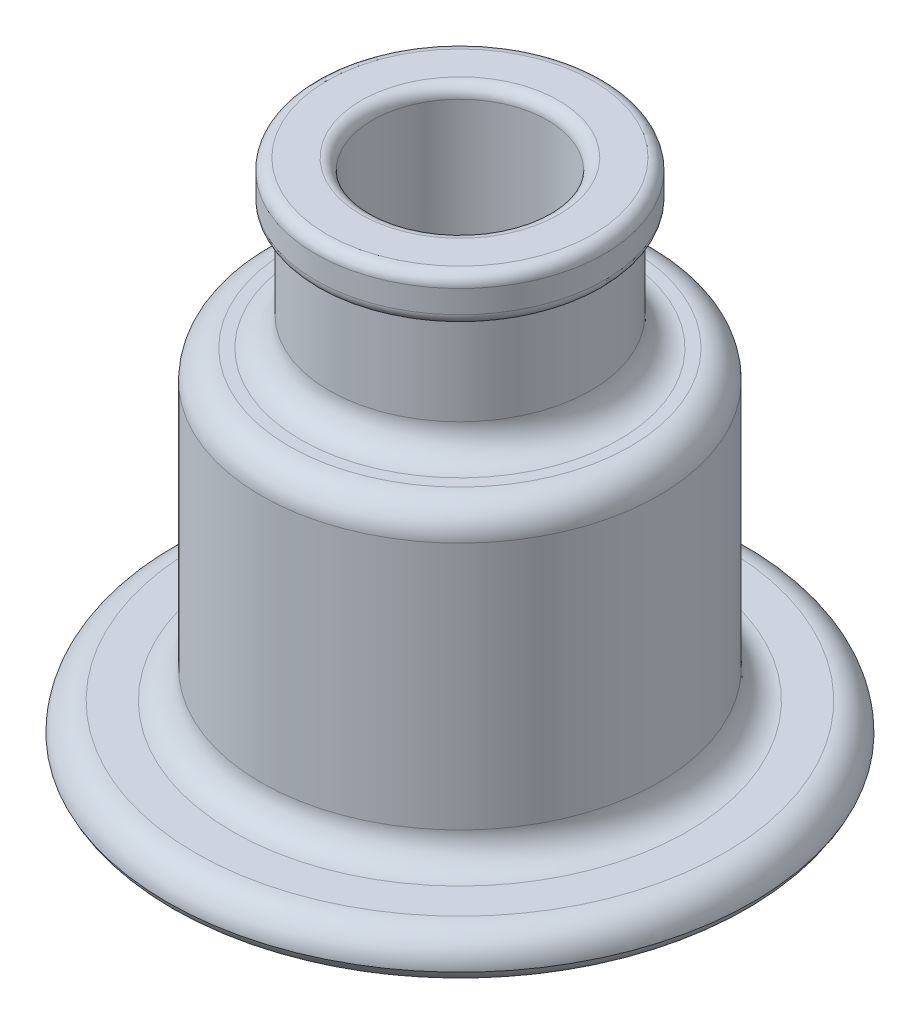
ISO-10303-21;
HEADER;
FILE_DESCRIPTION(('STEP AP214'),'2;1');
FILE_NAME('part.step','',(''),(''),'','','');
FILE_SCHEMA(('AUTOMOTIVE_DESIGN { 1 0 10303 214 1 1 1 1 }'));
ENDSEC;
DATA;
#1=APPLICATION_CONTEXT('core data for automotive mechanical design processes');
#2=APPLICATION_PROTOCOL_DEFINITION('international standard','automotive_design',2000,#1);
#3=PRODUCT_CONTEXT('',#1,'mechanical');
#4=PRODUCT('Part','Part','',(#3));
#5=PRODUCT_RELATED_PRODUCT_CATEGORY('part','',(#4));
#6=PRODUCT_DEFINITION_FORMATION('','',#4);
#7=PRODUCT_DEFINITION_CONTEXT('part definition',#1,'design');
#8=PRODUCT_DEFINITION('design','',#6,#7);
#9=PRODUCT_DEFINITION_SHAPE('','',#8);
#10=(LENGTH_UNIT() NAMED_UNIT(*) SI_UNIT(.MILLI.,.METRE.));
#11=(NAMED_UNIT(*) PLANE_ANGLE_UNIT() SI_UNIT($,.RADIAN.));
#12=(NAMED_UNIT(*) SI_UNIT($,.STERADIAN.) SOLID_ANGLE_UNIT());
#13=UNCERTAINTY_MEASURE_WITH_UNIT(LENGTH_MEASURE(1.E-05),#10,'distance_accuracy_value','');
#14=(GEOMETRIC_REPRESENTATION_CONTEXT(3) GLOBAL_UNCERTAINTY_ASSIGNED_CONTEXT((#13)) GLOBAL_UNIT_ASSIGNED_CONTEXT((#10,
#11,#12)) REPRESENTATION_CONTEXT('',''));
#15=CARTESIAN_POINT('',(0.,0.,0.));
#16=DIRECTION('',(0.,0.,1.));
#17=DIRECTION('',(1.,0.,0.));
#18=AXIS2_PLACEMENT_3D('',#15,#16,#17);
#19=CARTESIAN_POINT('',(0.,5.,0.));
#20=DIRECTION('',(0.,-1.,0.));
#21=DIRECTION('',(0.,0.,-1.));
#22=AXIS2_PLACEMENT_3D('',#19,#20,#21);
#23=CYLINDRICAL_SURFACE('',#22,32.);
#24=CARTESIAN_POINT('',(0.,2.,0.));
#25=DIRECTION('',(0.,1.,0.));
#26=DIRECTION('',(0.,0.,1.));
#27=AXIS2_PLACEMENT_3D('',#24,#25,#26);
#28=CIRCLE('',#27,32.);
#29=CARTESIAN_POINT('',(0.,2.,32.));
#30=VERTEX_POINT('',#29);
#31=EDGE_CURVE('E67',#30,#30,#28,.T.);
#32=ORIENTED_EDGE('',*,*,#31,.T.);
#33=EDGE_LOOP('',(#32));
#34=FACE_BOUND('',#33,.T.);
#35=CARTESIAN_POINT('',(0.,3.,0.));
#36=DIRECTION('',(0.,1.,0.));
#37=DIRECTION('',(0.,0.,1.));
#38=AXIS2_PLACEMENT_3D('',#35,#36,#37);
#39=CIRCLE('',#38,32.);
#40=CARTESIAN_POINT('',(0.,3.,32.));
#41=VERTEX_POINT('',#40);
#42=EDGE_CURVE('E66',#41,#41,#39,.F.);
#43=ORIENTED_EDGE('',*,*,#42,.T.);
#44=EDGE_LOOP('',(#43));
#45=FACE_BOUND('',#44,.T.);
#46=ADVANCED_FACE('F40',(#34,#45),#23,.T.);
#47=CARTESIAN_POINT('',(0.,0.,0.));
#48=DIRECTION('',(0.,1.,0.));
#49=DIRECTION('',(0.,0.,1.));
#50=AXIS2_PLACEMENT_3D('',#47,#48,#49);
#51=PLANE('',#50);
#52=CARTESIAN_POINT('',(0.,0.,0.));
#53=DIRECTION('',(0.,1.,0.));
#54=DIRECTION('',(0.,0.,1.));
#55=AXIS2_PLACEMENT_3D('',#52,#53,#54);
#56=CIRCLE('',#55,30.);
#57=CARTESIAN_POINT('',(0.,0.,30.));
#58=VERTEX_POINT('',#57);
#59=EDGE_CURVE('E64',#58,#58,#56,.F.);
#60=ORIENTED_EDGE('',*,*,#59,.T.);
#61=EDGE_LOOP('',(#60));
#62=FACE_BOUND('',#61,.T.);
#63=CARTESIAN_POINT('',(0.,0.,0.));
#64=DIRECTION('',(0.,-1.,0.));
#65=DIRECTION('',(0.,0.,-1.));
#66=AXIS2_PLACEMENT_3D('',#63,#64,#65);
#67=CIRCLE('',#66,25.);
#68=CARTESIAN_POINT('',(0.,0.,-25.));
#69=VERTEX_POINT('',#68);
#70=EDGE_CURVE('E106',#69,#69,#67,.T.);
#71=ORIENTED_EDGE('',*,*,#70,.F.);
#72=EDGE_LOOP('',(#71));
#73=FACE_BOUND('',#72,.T.);
#74=ADVANCED_FACE('F121',(#62,#73),#51,.F.);
#75=CARTESIAN_POINT('',(0.,13.,0.));
#76=DIRECTION('',(0.,1.,0.));
#77=DIRECTION('',(0.,0.,1.));
#78=AXIS2_PLACEMENT_3D('',#75,#76,#77);
#79=PLANE('',#78);
#80=CARTESIAN_POINT('',(0.,13.,0.));
#81=DIRECTION('',(0.,1.,0.));
#82=DIRECTION('',(0.,0.,1.));
#83=AXIS2_PLACEMENT_3D('',#80,#81,#82);
#84=CIRCLE('',#83,46.5);
#85=CARTESIAN_POINT('',(0.,13.,46.5));
#86=VERTEX_POINT('',#85);
#87=EDGE_CURVE('E81',#86,#86,#84,.T.);
#88=ORIENTED_EDGE('',*,*,#87,.T.);
#89=EDGE_LOOP('',(#88));
#90=FACE_BOUND('',#89,.T.);
#91=CARTESIAN_POINT('',(0.,13.,0.));
#92=DIRECTION('',(0.,1.,0.));
#93=DIRECTION('',(0.,0.,1.));
#94=AXIS2_PLACEMENT_3D('',#91,#92,#93);
#95=CIRCLE('',#94,40.);
#96=CARTESIAN_POINT('',(0.,13.,40.));
#97=VERTEX_POINT('',#96);
#98=EDGE_CURVE('E88',#97,#97,#95,.F.);
#99=ORIENTED_EDGE('',*,*,#98,.T.);
#100=EDGE_LOOP('',(#99));
#101=FACE_BOUND('',#100,.T.);
#102=ADVANCED_FACE('F126',(#90,#101),#79,.T.);
#103=CARTESIAN_POINT('',(0.,5.,0.));
#104=DIRECTION('',(0.,1.,0.));
#105=DIRECTION('',(0.,0.,1.));
#106=AXIS2_PLACEMENT_3D('',#103,#104,#105);
#107=PLANE('',#106);
#108=CARTESIAN_POINT('',(0.,5.,0.));
#109=DIRECTION('',(0.,1.,0.));
#110=DIRECTION('',(0.,0.,1.));
#111=AXIS2_PLACEMENT_3D('',#108,#109,#110);
#112=CIRCLE('',#111,34.);
#113=CARTESIAN_POINT('',(0.,5.,34.));
#114=VERTEX_POINT('',#113);
#115=EDGE_CURVE('E75',#114,#114,#112,.T.);
#116=ORIENTED_EDGE('',*,*,#115,.T.);
#117=EDGE_LOOP('',(#116));
#118=FACE_BOUND('',#117,.T.);
#119=CARTESIAN_POINT('',(0.,5.,0.));
#120=DIRECTION('',(0.,1.,0.));
#121=DIRECTION('',(0.,0.,1.));
#122=AXIS2_PLACEMENT_3D('',#119,#120,#121);
#123=CIRCLE('',#122,46.9174243050442);
#124=CARTESIAN_POINT('',(0.,5.,46.9174243050442));
#125=VERTEX_POINT('',#124);
#126=EDGE_CURVE('E74',#125,#125,#123,.F.);
#127=ORIENTED_EDGE('',*,*,#126,.T.);
#128=EDGE_LOOP('',(#127));
#129=FACE_BOUND('',#128,.T.);
#130=ADVANCED_FACE('F131',(#118,#129),#107,.F.);
#131=CARTESIAN_POINT('',(0.,66.7,0.));
#132=DIRECTION('',(0.,-1.,0.));
#133=DIRECTION('',(0.,0.,-1.));
#134=AXIS2_PLACEMENT_3D('',#131,#132,#133);
#135=CYLINDRICAL_SURFACE('',#134,35.);
#136=CARTESIAN_POINT('',(0.,61.7,0.));
#137=DIRECTION('',(0.,1.,0.));
#138=DIRECTION('',(0.,0.,1.));
#139=AXIS2_PLACEMENT_3D('',#136,#137,#138);
#140=CIRCLE('',#139,35.);
#141=CARTESIAN_POINT('',(0.,61.7,-35.));
#142=VERTEX_POINT('',#141);
#143=EDGE_CURVE('E83',#142,#142,#140,.F.);
#144=CARTESIAN_POINT('',(0.,18.,0.));
#145=DIRECTION('',(0.,1.,0.));
#146=DIRECTION('',(0.,0.,1.));
#147=AXIS2_PLACEMENT_3D('',#144,#145,#146);
#148=CIRCLE('',#147,35.);
#149=CARTESIAN_POINT('',(0.,18.,-35.));
#150=VERTEX_POINT('',#149);
#151=EDGE_CURVE('E92',#150,#150,#148,.T.);
#152=CARTESIAN_POINT('',(0.,61.7,-35.));
#153=CARTESIAN_POINT('',(0.,61.2447916666667,-35.));
#154=CARTESIAN_POINT('',(0.,60.7895833333333,-35.));
#155=CARTESIAN_POINT('',(0.,59.8791666666667,-35.));
#156=CARTESIAN_POINT('',(0.,59.4239583333333,-35.));
#157=CARTESIAN_POINT('',(0.,58.5135416666667,-35.));
#158=CARTESIAN_POINT('',(0.,58.0583333333333,-35.));
#159=CARTESIAN_POINT('',(0.,57.1479166666667,-35.));
#160=CARTESIAN_POINT('',(0.,56.6927083333333,-35.));
#161=CARTESIAN_POINT('',(0.,55.7822916666667,-35.));
#162=CARTESIAN_POINT('',(0.,55.3270833333333,-35.));
#163=CARTESIAN_POINT('',(0.,54.4166666666667,-35.));
#164=CARTESIAN_POINT('',(0.,53.9614583333333,-35.));
#165=CARTESIAN_POINT('',(0.,53.0510416666667,-35.));
#166=CARTESIAN_POINT('',(0.,52.5958333333333,-35.));
#167=CARTESIAN_POINT('',(0.,51.6854166666667,-35.));
#168=CARTESIAN_POINT('',(0.,51.2302083333333,-35.));
#169=CARTESIAN_POINT('',(0.,50.3197916666667,-35.));
#170=CARTESIAN_POINT('',(0.,49.8645833333333,-35.));
#171=CARTESIAN_POINT('',(0.,48.9541666666667,-35.));
#172=CARTESIAN_POINT('',(0.,48.4989583333333,-35.));
#173=CARTESIAN_POINT('',(0.,47.5885416666667,-35.));
#174=CARTESIAN_POINT('',(0.,47.1333333333333,-35.));
#175=CARTESIAN_POINT('',(0.,46.2229166666667,-35.));
#176=CARTESIAN_POINT('',(0.,45.7677083333333,-35.));
#177=CARTESIAN_POINT('',(0.,44.8572916666667,-35.));
#178=CARTESIAN_POINT('',(0.,44.4020833333333,-35.));
#179=CARTESIAN_POINT('',(0.,43.4916666666667,-35.));
#180=CARTESIAN_POINT('',(0.,43.0364583333333,-35.));
#181=CARTESIAN_POINT('',(0.,42.1260416666667,-35.));
#182=CARTESIAN_POINT('',(0.,41.6708333333333,-35.));
#183=CARTESIAN_POINT('',(0.,40.7604166666667,-35.));
#184=CARTESIAN_POINT('',(0.,40.3052083333333,-35.));
#185=CARTESIAN_POINT('',(0.,39.3947916666667,-35.));
#186=CARTESIAN_POINT('',(0.,38.9395833333333,-35.));
#187=CARTESIAN_POINT('',(0.,38.0291666666667,-35.));
#188=CARTESIAN_POINT('',(0.,37.5739583333333,-35.));
#189=CARTESIAN_POINT('',(0.,36.6635416666667,-35.));
#190=CARTESIAN_POINT('',(0.,36.2083333333333,-35.));
#191=CARTESIAN_POINT('',(0.,35.2979166666667,-35.));
#192=CARTESIAN_POINT('',(0.,34.8427083333333,-35.));
#193=CARTESIAN_POINT('',(0.,33.9322916666667,-35.));
#194=CARTESIAN_POINT('',(0.,33.4770833333333,-35.));
#195=CARTESIAN_POINT('',(0.,32.5666666666667,-35.));
#196=CARTESIAN_POINT('',(0.,32.1114583333333,-35.));
#197=CARTESIAN_POINT('',(0.,31.2010416666667,-35.));
#198=CARTESIAN_POINT('',(0.,30.7458333333333,-35.));
#199=CARTESIAN_POINT('',(0.,29.8354166666667,-35.));
#200=CARTESIAN_POINT('',(0.,29.3802083333333,-35.));
#201=CARTESIAN_POINT('',(0.,28.4697916666667,-35.));
#202=CARTESIAN_POINT('',(0.,28.0145833333333,-35.));
#203=CARTESIAN_POINT('',(0.,27.1041666666667,-35.));
#204=CARTESIAN_POINT('',(0.,26.6489583333333,-35.));
#205=CARTESIAN_POINT('',(0.,25.7385416666667,-35.));
#206=CARTESIAN_POINT('',(0.,25.2833333333333,-35.));
#207=CARTESIAN_POINT('',(0.,24.3729166666667,-35.));
#208=CARTESIAN_POINT('',(0.,23.9177083333333,-35.));
#209=CARTESIAN_POINT('',(0.,23.0072916666667,-35.));
#210=CARTESIAN_POINT('',(0.,22.5520833333333,-35.));
#211=CARTESIAN_POINT('',(0.,21.6416666666667,-35.));
#212=CARTESIAN_POINT('',(0.,21.1864583333333,-35.));
#213=CARTESIAN_POINT('',(0.,20.2760416666667,-35.));
#214=CARTESIAN_POINT('',(0.,19.8208333333333,-35.));
#215=CARTESIAN_POINT('',(0.,18.9104166666667,-35.));
#216=CARTESIAN_POINT('',(0.,18.4552083333333,-35.));
#217=CARTESIAN_POINT('',(0.,18.,-35.));
#218=B_SPLINE_CURVE_WITH_KNOTS('',3,(#152,#153,#154,#155,#156,#157,#158,#159,#160,#161,#162,
#163,#164,#165,#166,#167,#168,#169,#170,#171,#172,#173,#174,#175,#176,#177,#178,#179,#180,#181,
#182,#183,#184,#185,#186,#187,#188,#189,#190,#191,#192,#193,#194,#195,#196,#197,#198,#199,#200,
#201,#202,#203,#204,#205,#206,#207,#208,#209,#210,#211,#212,#213,#214,#215,#216,#217),
.UNSPECIFIED.,.F.,.F.,(4,2,2,2,2,2,2,2,2,2,2,2,2,2,2,2,2,2,2,2,2,2,2,2,2,2,2,2,2,2,2,2,4),(0.,
1.365625,2.73125,4.09687500000001,5.4625,6.828125,8.19375000000001,9.559375,10.925,12.290625,
13.65625,15.021875,16.3875,17.753125,19.11875,20.484375,21.85,23.215625,24.58125,25.946875,
27.3125,28.678125,30.04375,31.409375,32.775,34.140625,35.50625,36.871875,38.2375,39.603125,
40.96875,42.334375,43.7),.UNSPECIFIED.);
#219=EDGE_CURVE('BSEAM214',#142,#150,#218,.T.);
#220=ORIENTED_EDGE('',*,*,#143,.T.);
#221=ORIENTED_EDGE('',*,*,#151,.T.);
#222=ORIENTED_EDGE('',*,*,#219,.T.);
#223=ORIENTED_EDGE('',*,*,#219,.F.);
#224=EDGE_LOOP('',(#220,#222,#221,#223));
#225=FACE_BOUND('',#224,.T.);
#226=ADVANCED_FACE('F214',(#225),#135,.T.);
#227=CARTESIAN_POINT('',(0.,66.7,0.));
#228=DIRECTION('',(0.,1.,0.));
#229=DIRECTION('',(0.,0.,1.));
#230=AXIS2_PLACEMENT_3D('',#227,#228,#229);
#231=PLANE('',#230);
#232=CARTESIAN_POINT('',(0.,66.7,0.));
#233=DIRECTION('',(0.,1.,0.));
#234=DIRECTION('',(0.,0.,1.));
#235=AXIS2_PLACEMENT_3D('',#232,#233,#234);
#236=CIRCLE('',#235,30.);
#237=CARTESIAN_POINT('',(0.,66.7,30.));
#238=VERTEX_POINT('',#237);
#239=EDGE_CURVE('E90',#238,#238,#236,.T.);
#240=ORIENTED_EDGE('',*,*,#239,.T.);
#241=EDGE_LOOP('',(#240));
#242=FACE_BOUND('',#241,.T.);
#243=CARTESIAN_POINT('',(0.,66.7,0.));
#244=DIRECTION('',(0.,1.,0.));
#245=DIRECTION('',(0.,0.,1.));
#246=AXIS2_PLACEMENT_3D('',#243,#244,#245);
#247=CIRCLE('',#246,28.);
#248=CARTESIAN_POINT('',(0.,66.7,28.));
#249=VERTEX_POINT('',#248);
#250=EDGE_CURVE('E98',#249,#249,#247,.F.);
#251=ORIENTED_EDGE('',*,*,#250,.T.);
#252=EDGE_LOOP('',(#251));
#253=FACE_BOUND('',#252,.T.);
#254=ADVANCED_FACE('F209',(#242,#253),#231,.T.);
#255=CARTESIAN_POINT('',(0.,87.7,0.));
#256=DIRECTION('',(0.,-1.,0.));
#257=DIRECTION('',(0.,0.,-1.));
#258=AXIS2_PLACEMENT_3D('',#255,#256,#257);
#259=CYLINDRICAL_SURFACE('',#258,23.);
#260=CARTESIAN_POINT('',(0.,71.7,0.));
#261=DIRECTION('',(0.,1.,0.));
#262=DIRECTION('',(0.,0.,1.));
#263=AXIS2_PLACEMENT_3D('',#260,#261,#262);
#264=CIRCLE('',#263,23.);
#265=CARTESIAN_POINT('',(0.,71.7,23.));
#266=VERTEX_POINT('',#265);
#267=EDGE_CURVE('E100',#266,#266,#264,.T.);
#268=ORIENTED_EDGE('',*,*,#267,.T.);
#269=EDGE_LOOP('',(#268));
#270=FACE_BOUND('',#269,.T.);
#271=CARTESIAN_POINT('',(0.,87.7,0.));
#272=DIRECTION('',(0.,1.,0.));
#273=DIRECTION('',(0.,0.,1.));
#274=AXIS2_PLACEMENT_3D('',#271,#272,#273);
#275=CIRCLE('',#274,23.);
#276=CARTESIAN_POINT('',(0.,87.7,23.));
#277=VERTEX_POINT('',#276);
#278=EDGE_CURVE('E105',#277,#277,#275,.T.);
#279=ORIENTED_EDGE('',*,*,#278,.F.);
#280=EDGE_LOOP('',(#279));
#281=FACE_BOUND('',#280,.T.);
#282=ADVANCED_FACE('F210',(#270,#281),#259,.T.);
#283=CARTESIAN_POINT('',(0.,95.7,0.));
#284=DIRECTION('',(0.,-1.,0.));
#285=DIRECTION('',(0.,0.,-1.));
#286=AXIS2_PLACEMENT_3D('',#283,#284,#285);
#287=CYLINDRICAL_SURFACE('',#286,25.4);
#288=CARTESIAN_POINT('',(0.,89.7,0.));
#289=DIRECTION('',(0.,1.,0.));
#290=DIRECTION('',(0.,0.,1.));
#291=AXIS2_PLACEMENT_3D('',#288,#289,#290);
#292=CIRCLE('',#291,25.4);
#293=CARTESIAN_POINT('',(0.,89.7,25.4));
#294=VERTEX_POINT('',#293);
#295=EDGE_CURVE('E42',#294,#294,#292,.T.);
#296=ORIENTED_EDGE('',*,*,#295,.T.);
#297=EDGE_LOOP('',(#296));
#298=FACE_BOUND('',#297,.T.);
#299=CARTESIAN_POINT('',(0.,93.7,0.));
#300=DIRECTION('',(0.,1.,0.));
#301=DIRECTION('',(0.,0.,1.));
#302=AXIS2_PLACEMENT_3D('',#299,#300,#301);
#303=CIRCLE('',#302,25.4);
#304=CARTESIAN_POINT('',(0.,93.7,25.4));
#305=VERTEX_POINT('',#304);
#306=EDGE_CURVE('E48',#305,#305,#303,.F.);
#307=ORIENTED_EDGE('',*,*,#306,.T.);
#308=EDGE_LOOP('',(#307));
#309=FACE_BOUND('',#308,.T.);
#310=ADVANCED_FACE('F190',(#298,#309),#287,.T.);
#311=CARTESIAN_POINT('',(0.,95.7,0.));
#312=DIRECTION('',(0.,1.,0.));
#313=DIRECTION('',(0.,0.,1.));
#314=AXIS2_PLACEMENT_3D('',#311,#312,#313);
#315=PLANE('',#314);
#316=CARTESIAN_POINT('',(0.,95.7,0.));
#317=DIRECTION('',(0.,1.,0.));
#318=DIRECTION('',(0.,0.,1.));
#319=AXIS2_PLACEMENT_3D('',#316,#317,#318);
#320=CIRCLE('',#319,23.4);
#321=CARTESIAN_POINT('',(0.,95.7,23.4));
#322=VERTEX_POINT('',#321);
#323=EDGE_CURVE('E55',#322,#322,#320,.T.);
#324=ORIENTED_EDGE('',*,*,#323,.T.);
#325=EDGE_LOOP('',(#324));
#326=FACE_BOUND('',#325,.T.);
#327=CARTESIAN_POINT('',(0.,95.7,0.));
#328=DIRECTION('',(0.,1.,0.));
#329=DIRECTION('',(0.,0.,1.));
#330=AXIS2_PLACEMENT_3D('',#327,#328,#329);
#331=CIRCLE('',#330,17.4);
#332=CARTESIAN_POINT('',(0.,95.7,17.4));
#333=VERTEX_POINT('',#332);
#334=EDGE_CURVE('E60',#333,#333,#331,.F.);
#335=ORIENTED_EDGE('',*,*,#334,.T.);
#336=EDGE_LOOP('',(#335));
#337=FACE_BOUND('',#336,.T.);
#338=ADVANCED_FACE('F184',(#326,#337),#315,.T.);
#339=CARTESIAN_POINT('',(0.,87.7,0.));
#340=DIRECTION('',(0.,1.,0.));
#341=DIRECTION('',(0.,0.,1.));
#342=AXIS2_PLACEMENT_3D('',#339,#340,#341);
#343=PLANE('',#342);
#344=CARTESIAN_POINT('',(0.,87.7,0.));
#345=DIRECTION('',(0.,1.,0.));
#346=DIRECTION('',(0.,0.,1.));
#347=AXIS2_PLACEMENT_3D('',#344,#345,#346);
#348=CIRCLE('',#347,23.4);
#349=CARTESIAN_POINT('',(0.,87.7,23.4));
#350=VERTEX_POINT('',#349);
#351=EDGE_CURVE('E10',#350,#350,#348,.F.);
#352=ORIENTED_EDGE('',*,*,#351,.T.);
#353=EDGE_LOOP('',(#352));
#354=FACE_BOUND('',#353,.T.);
#355=ORIENTED_EDGE('',*,*,#278,.T.);
#356=EDGE_LOOP('',(#355));
#357=FACE_BOUND('',#356,.T.);
#358=ADVANCED_FACE('F119',(#354,#357),#343,.F.);
#359=CARTESIAN_POINT('',(0.,66.,0.));
#360=DIRECTION('',(0.,-1.,0.));
#361=DIRECTION('',(0.,0.,-1.));
#362=AXIS2_PLACEMENT_3D('',#359,#360,#361);
#363=CYLINDRICAL_SURFACE('',#362,25.);
#364=CARTESIAN_POINT('',(0.,66.,0.));
#365=DIRECTION('',(0.,-1.,0.));
#366=DIRECTION('',(0.,0.,-1.));
#367=AXIS2_PLACEMENT_3D('',#364,#365,#366);
#368=CIRCLE('',#367,25.);
#369=CARTESIAN_POINT('',(0.,66.,-25.));
#370=VERTEX_POINT('',#369);
#371=EDGE_CURVE('E107',#370,#370,#368,.T.);
#372=ORIENTED_EDGE('',*,*,#371,.F.);
#373=EDGE_LOOP('',(#372));
#374=FACE_BOUND('',#373,.T.);
#375=ORIENTED_EDGE('',*,*,#70,.T.);
#376=EDGE_LOOP('',(#375));
#377=FACE_BOUND('',#376,.T.);
#378=ADVANCED_FACE('F120',(#374,#377),#363,.F.);
#379=CARTESIAN_POINT('',(0.,66.,0.));
#380=DIRECTION('',(0.,-1.,0.));
#381=DIRECTION('',(0.,0.,-1.));
#382=AXIS2_PLACEMENT_3D('',#379,#380,#381);
#383=PLANE('',#382);
#384=CARTESIAN_POINT('',(0.,66.,0.));
#385=DIRECTION('',(0.,-1.,0.));
#386=DIRECTION('',(0.,0.,-1.));
#387=AXIS2_PLACEMENT_3D('',#384,#385,#386);
#388=CIRCLE('',#387,15.4);
#389=CARTESIAN_POINT('',(0.,66.,-15.4));
#390=VERTEX_POINT('',#389);
#391=EDGE_CURVE('E101',#390,#390,#388,.T.);
#392=ORIENTED_EDGE('',*,*,#391,.F.);
#393=EDGE_LOOP('',(#392));
#394=FACE_BOUND('',#393,.T.);
#395=ORIENTED_EDGE('',*,*,#371,.T.);
#396=EDGE_LOOP('',(#395));
#397=FACE_BOUND('',#396,.T.);
#398=ADVANCED_FACE('F114',(#394,#397),#383,.T.);
#399=CARTESIAN_POINT('',(0.,29.7,0.));
#400=DIRECTION('',(0.,1.,0.));
#401=DIRECTION('',(0.,0.,1.));
#402=AXIS2_PLACEMENT_3D('',#399,#400,#401);
#403=CYLINDRICAL_SURFACE('',#402,15.4);
#404=CARTESIAN_POINT('',(0.,93.7,0.));
#405=DIRECTION('',(0.,1.,0.));
#406=DIRECTION('',(0.,0.,1.));
#407=AXIS2_PLACEMENT_3D('',#404,#405,#406);
#408=CIRCLE('',#407,15.4);
#409=CARTESIAN_POINT('',(0.,93.7,15.4));
#410=VERTEX_POINT('',#409);
#411=EDGE_CURVE('E58',#410,#410,#408,.T.);
#412=ORIENTED_EDGE('',*,*,#411,.T.);
#413=EDGE_LOOP('',(#412));
#414=FACE_BOUND('',#413,.T.);
#415=ORIENTED_EDGE('',*,*,#391,.T.);
#416=EDGE_LOOP('',(#415));
#417=FACE_BOUND('',#416,.T.);
#418=ADVANCED_FACE('F143',(#414,#417),#403,.F.);
#419=CARTESIAN_POINT('',(0.,71.7,0.));
#420=DIRECTION('',(0.,1.,0.));
#421=DIRECTION('',(0.,0.,1.));
#422=AXIS2_PLACEMENT_3D('',#419,#420,#421);
#423=TOROIDAL_SURFACE('',#422,28.,5.);
#424=ORIENTED_EDGE('',*,*,#250,.F.);
#425=EDGE_LOOP('',(#424));
#426=FACE_BOUND('',#425,.T.);
#427=ORIENTED_EDGE('',*,*,#267,.F.);
#428=EDGE_LOOP('',(#427));
#429=FACE_BOUND('',#428,.T.);
#430=ADVANCED_FACE('F142',(#426,#429),#423,.F.);
#431=CARTESIAN_POINT('',(0.,18.,0.));
#432=DIRECTION('',(0.,1.,0.));
#433=DIRECTION('',(0.,0.,1.));
#434=AXIS2_PLACEMENT_3D('',#431,#432,#433);
#435=TOROIDAL_SURFACE('',#434,40.,5.);
#436=ORIENTED_EDGE('',*,*,#98,.F.);
#437=EDGE_LOOP('',(#436));
#438=FACE_BOUND('',#437,.T.);
#439=ORIENTED_EDGE('',*,*,#151,.F.);
#440=EDGE_LOOP('',(#439));
#441=FACE_BOUND('',#440,.T.);
#442=ADVANCED_FACE('F144',(#438,#441),#435,.F.);
#443=CARTESIAN_POINT('',(0.,61.7,0.));
#444=DIRECTION('',(0.,1.,0.));
#445=DIRECTION('',(0.,0.,1.));
#446=AXIS2_PLACEMENT_3D('',#443,#444,#445);
#447=TOROIDAL_SURFACE('',#446,30.,5.);
#448=ORIENTED_EDGE('',*,*,#143,.F.);
#449=EDGE_LOOP('',(#448));
#450=FACE_BOUND('',#449,.T.);
#451=ORIENTED_EDGE('',*,*,#239,.F.);
#452=EDGE_LOOP('',(#451));
#453=FACE_BOUND('',#452,.T.);
#454=ADVANCED_FACE('F148',(#450,#453),#447,.T.);
#455=CARTESIAN_POINT('',(0.,8.,0.));
#456=DIRECTION('',(0.,1.,0.));
#457=DIRECTION('',(0.,0.,1.));
#458=AXIS2_PLACEMENT_3D('',#455,#456,#457);
#459=TOROIDAL_SURFACE('',#458,46.5,5.);
#460=CARTESIAN_POINT('',(0.,8.,0.));
#461=DIRECTION('',(0.,1.,0.));
#462=DIRECTION('',(0.,0.,1.));
#463=AXIS2_PLACEMENT_3D('',#460,#461,#462);
#464=CIRCLE('',#463,51.5);
#465=CARTESIAN_POINT('',(0.,8.,51.5));
#466=VERTEX_POINT('',#465);
#467=EDGE_CURVE('E76',#466,#466,#464,.F.);
#468=ORIENTED_EDGE('',*,*,#467,.F.);
#469=EDGE_LOOP('',(#468));
#470=FACE_BOUND('',#469,.T.);
#471=ORIENTED_EDGE('',*,*,#87,.F.);
#472=EDGE_LOOP('',(#471));
#473=FACE_BOUND('',#472,.T.);
#474=ADVANCED_FACE('F154',(#470,#473),#459,.T.);
#475=CARTESIAN_POINT('',(0.,10.,0.));
#476=DIRECTION('',(0.,-1.,0.));
#477=DIRECTION('',(0.,0.,-1.));
#478=AXIS2_PLACEMENT_3D('',#475,#476,#477);
#479=TOROIDAL_SURFACE('',#478,46.9174243050442,5.);
#480=ORIENTED_EDGE('',*,*,#126,.F.);
#481=EDGE_LOOP('',(#480));
#482=FACE_BOUND('',#481,.T.);
#483=ORIENTED_EDGE('',*,*,#467,.T.);
#484=EDGE_LOOP('',(#483));
#485=FACE_BOUND('',#484,.T.);
#486=ADVANCED_FACE('F160',(#482,#485),#479,.T.);
#487=CARTESIAN_POINT('',(0.,3.,0.));
#488=DIRECTION('',(0.,1.,0.));
#489=DIRECTION('',(0.,0.,1.));
#490=AXIS2_PLACEMENT_3D('',#487,#488,#489);
#491=TOROIDAL_SURFACE('',#490,34.,2.);
#492=ORIENTED_EDGE('',*,*,#42,.F.);
#493=EDGE_LOOP('',(#492));
#494=FACE_BOUND('',#493,.T.);
#495=ORIENTED_EDGE('',*,*,#115,.F.);
#496=EDGE_LOOP('',(#495));
#497=FACE_BOUND('',#496,.T.);
#498=ADVANCED_FACE('F163',(#494,#497),#491,.F.);
#499=CARTESIAN_POINT('',(0.,2.,0.));
#500=DIRECTION('',(0.,1.,0.));
#501=DIRECTION('',(0.,0.,1.));
#502=AXIS2_PLACEMENT_3D('',#499,#500,#501);
#503=TOROIDAL_SURFACE('',#502,30.,2.);
#504=ORIENTED_EDGE('',*,*,#59,.F.);
#505=EDGE_LOOP('',(#504));
#506=FACE_BOUND('',#505,.T.);
#507=ORIENTED_EDGE('',*,*,#31,.F.);
#508=EDGE_LOOP('',(#507));
#509=FACE_BOUND('',#508,.T.);
#510=ADVANCED_FACE('F164',(#506,#509),#503,.T.);
#511=CARTESIAN_POINT('',(0.,93.7,0.));
#512=DIRECTION('',(0.,1.,0.));
#513=DIRECTION('',(0.,0.,1.));
#514=AXIS2_PLACEMENT_3D('',#511,#512,#513);
#515=TOROIDAL_SURFACE('',#514,17.4,2.);
#516=ORIENTED_EDGE('',*,*,#334,.F.);
#517=EDGE_LOOP('',(#516));
#518=FACE_BOUND('',#517,.T.);
#519=ORIENTED_EDGE('',*,*,#411,.F.);
#520=EDGE_LOOP('',(#519));
#521=FACE_BOUND('',#520,.T.);
#522=ADVANCED_FACE('F166',(#518,#521),#515,.T.);
#523=CARTESIAN_POINT('',(0.,93.7,0.));
#524=DIRECTION('',(0.,1.,0.));
#525=DIRECTION('',(0.,0.,1.));
#526=AXIS2_PLACEMENT_3D('',#523,#524,#525);
#527=TOROIDAL_SURFACE('',#526,23.4,2.);
#528=ORIENTED_EDGE('',*,*,#306,.F.);
#529=EDGE_LOOP('',(#528));
#530=FACE_BOUND('',#529,.T.);
#531=ORIENTED_EDGE('',*,*,#323,.F.);
#532=EDGE_LOOP('',(#531));
#533=FACE_BOUND('',#532,.T.);
#534=ADVANCED_FACE('F171',(#530,#533),#527,.T.);
#535=CARTESIAN_POINT('',(0.,89.7,0.));
#536=DIRECTION('',(0.,1.,0.));
#537=DIRECTION('',(0.,0.,1.));
#538=AXIS2_PLACEMENT_3D('',#535,#536,#537);
#539=TOROIDAL_SURFACE('',#538,23.4,2.);
#540=ORIENTED_EDGE('',*,*,#351,.F.);
#541=EDGE_LOOP('',(#540));
#542=FACE_BOUND('',#541,.T.);
#543=ORIENTED_EDGE('',*,*,#295,.F.);
#544=EDGE_LOOP('',(#543));
#545=FACE_BOUND('',#544,.T.);
#546=ADVANCED_FACE('F39',(#542,#545),#539,.T.);
#547=CLOSED_SHELL('',(#46,#74,#102,#130,#226,#254,#282,#310,#338,#358,#378,#398,#418,#430,#442,
#454,#474,#486,#498,#510,#522,#534,#546));
#548=MANIFOLD_SOLID_BREP('B2',#547);
#549=ADVANCED_BREP_SHAPE_REPRESENTATION('',(#18,#548),#14);
#550=SHAPE_DEFINITION_REPRESENTATION(#9,#549);
ENDSEC;
END-ISO-10303-21;
